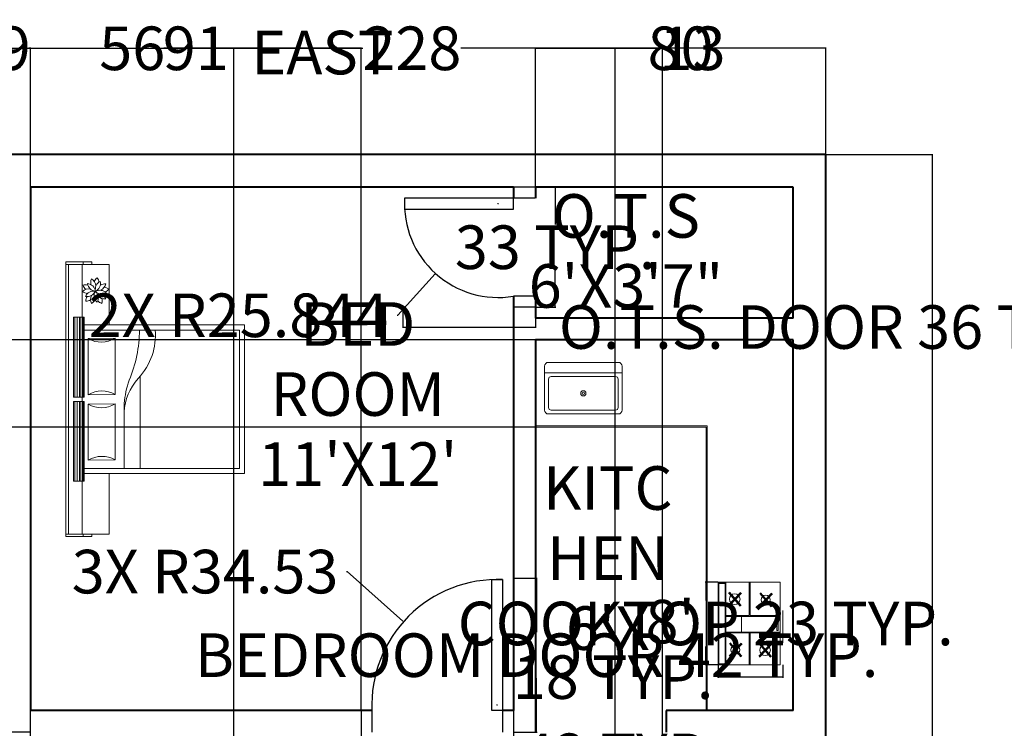
# Model space of a CAD drawing. Units: inches. Extents: x -124 to 612, y -69 to 524.
# Tile 6 of 9: x 16 to 287, y 329 to 524. Entities that reach past the tile are written whole.
import ezdxf
from ezdxf.enums import TextEntityAlignment as Align

# ---------------------------------------------------------------- set-up
doc = ezdxf.new("R2010")
doc.units = ezdxf.units.IN
doc.header["$MEASUREMENT"] = 0
for name, color, linetype, lineweight in [('A-ANNO-DIMS', 2, 'Continuous', 18), ('A-ANNO-TEXT', 1, 'Continuous', 18), ('A-AREA-IDEN', 1, 'Continuous', 18), ('A-DOOR', 4, 'Continuous', 25), ('A-EQPM', 9, 'Continuous', 18), ('A-FLOR-CASE', 8, 'Continuous', 18), ('A-FLOR-FIXT', 9, 'Continuous', 18), ('A-FURN', 8, 'Continuous', 18), ('A-WALL', 7, 'Continuous', 40)]:
    doc.layers.add(name, color=color, linetype=linetype, lineweight=lineweight)
doc.styles.add('ATTR', font='romans.shx', dxfattribs={"width": 0.8, "height": 1.075})
doc.styles.get("Standard").update_dxf_attribs({"font": 'arial.ttf'})
doc.dimstyles.get("Standard").update_dxf_attribs({"dimtxt": 12, "dimasz": 0.18, "dimexe": 0.18, "dimexo": 0.0625, "dimgap": 0.09, "dimtad": 0, "dimtih": 1, "dimtoh": 1, "dimdec": 0, "dimzin": 0, "dimdsep": 46, "dimlunit": 4, "dimtxsty": 'Standard', "dimcen": 0.09, "dimadec": 0, "dimazin": 0, "dimtfac": 1, "dimtdec": 0, "dimtofl": 0, "dimtmove": 0, "dimatfit": 3, "dimfxl": 1, "dimtolj": 1, "dimtzin": 0, "dimarcsym": 0})

# ---------------------------------------------------------------- blocks, each defined once
blk = doc.blocks.new('A$C7BDD1693')
for p, q in [((0, 2.068), (0, 1.768)), ((0, 2.068), (1.615, 2.068)), ((0.03, 1.768), (0.03, 2.068)), ((1.615, 2.068), (2.54, 2.068)), ((2.54, 2.068), (3.18, 2.068)), ((3.15, 1.768), (3.15, 2.068)), ((3.18, 2.068), (3.18, 1.768)), ((0.03, 2.038), (0.64, 2.038)), ((0.64, 2.038), (1.565, 2.038)), ((0.64, 1.978), (1.565, 1.978)), ((0.64, 1.978), (0.64, 1.858)), ((0.64, 1.963), (1.565, 1.963)), ((1.565, 2.038), (1.615, 2.038)), ((1.565, 1.978), (1.565, 1.858)), ((1.615, 2.038), (2.54, 2.038)), ((1.615, 1.978), (1.615, 1.858)), ((1.615, 1.978), (2.54, 1.978)), ((1.615, 1.963), (2.54, 1.963)), ((3.15, 2.038), (2.54, 2.038)), ((2.54, 1.978), (2.54, 1.858)), ((0.03, 1.868), (0, 1.868)), ((0.03, 1.88), (0.64, 1.88)), ((0.64, 1.937), (1.565, 1.937)), ((0.64, 1.912), (1.565, 1.912)), ((0.64, 1.893), (1.565, 1.893)), ((0.64, 1.877), (1.565, 1.877)), ((0.64, 1.866), (1.565, 1.866)), ((0.64, 1.858), (1.565, 1.858)), ((0.73, 1.568), (0.73, 1.858)), ((0.79, 1.858), (0.79, 0.06)), ((1.565, 1.88), (1.615, 1.88)), ((1.615, 1.937), (2.54, 1.937)), ((1.615, 1.912), (2.54, 1.912)), ((1.615, 1.893), (2.54, 1.893)), ((1.615, 1.877), (2.54, 1.877)), ((1.615, 1.866), (2.54, 1.866)), ((1.615, 1.858), (2.54, 1.858)), ((2.39, 1.858), (2.39, 0.06)), ((2.45, 1.568), (2.45, 1.858)), ((3.15, 1.88), (2.54, 1.88)), ((3.15, 1.868), (3.18, 1.868)), ((0, 1.768), (0.03, 1.768)), ((0.03, 1.768), (0.03, 1.568)), ((0.03, 1.768), (0.03, 1.568)), ((1.533, 1.81), (0.883, 1.81)), ((0.883, 1.81), (0.887, 1.498)), ((1.537, 1.498), (1.533, 1.81)), ((2.291, 1.81), (1.641, 1.81)), ((1.641, 1.81), (1.646, 1.498)), ((2.296, 1.498), (2.291, 1.81)), ((3.15, 1.568), (3.15, 1.768)), ((3.18, 1.768), (3.15, 1.768)), ((0.03, 1.568), (0.73, 1.568)), ((0.73, 1.568), (0.73, 0)), ((0.887, 1.498), (1.537, 1.498)), ((1.646, 1.498), (2.296, 1.498)), ((3.15, 1.568), (2.45, 1.568)), ((2.45, 1.568), (2.45, 0)), ((1.54, 1.392), (0.79, 1.392)), ((1.848, 1.209), (0.79, 1.209)), ((0.73, 0), (2.45, 0)), ((0.79, 0.06), (2.39, 0.06))]:
    blk.add_line(p, q)
for centre, radius, start, end in [((2.879, 1.849), 0.155, 184.2105, 205.3514), ((2.726, 1.74), 0.0968, 57.5086, 91.2476), ((2.884, 1.823), 0.106, 170.7761, 244.5159), ((2.743, 1.749), 0.098, 347.0447, 68.2473), ((2.938, 1.802), 0.125, 143.1301, 173.4932), ((2.751, 1.802), 0.115, 351.1324, 40.6013), ((2.967, 1.726), 0.155, 112.2105, 133.3514), ((2.817, 1.838), 0.0968, 345.5086, 19.2476), ((0.626, 1.65), 0.303, 329.8722, 31.8713), ((1.794, 1.658), 0.303, 149.8722, 211.8713), ((1.384, 1.65), 0.303, 329.8722, 31.8713), ((2.553, 1.658), 0.303, 149.8722, 211.8713), ((2.74, 1.667), 0.115, 63.1324, 112.6013), ((2.798, 1.845), 0.125, 215.1301, 245.4931), ((2.788, 1.643), 0.098, 59.0447, 140.2473), ((2.761, 1.8), 0.106, 242.7761, 316.5159), ((2.903, 1.653), 0.098, 131.0447, 212.2473), ((2.745, 1.676), 0.106, 314.7761, 28.5159), ((2.944, 1.713), 0.106, 98.7761, 172.5159), ((2.83, 1.825), 0.098, 275.0447, 356.2473), ((2.858, 1.622), 0.106, 26.7761, 100.5159), ((2.929, 1.765), 0.098, 203.0447, 284.2473), ((2.883, 1.833), 0.115, 279.1324, 328.6013), ((2.941, 1.655), 0.125, 71.1301, 101.4931), ((2.877, 1.605), 0.155, 40.2105, 61.3514), ((2.791, 1.624), 0.0968, 129.5086, 163.2476), ((2.735, 1.803), 0.155, 256.2105, 277.3514), ((2.865, 1.615), 0.115, 135.1324, 184.6013), ((2.713, 1.725), 0.125, 287.1301, 317.4932), ((2.921, 1.65), 0.0968, 201.5086, 235.2476), ((2.953, 1.718), 0.115, 207.1324, 256.6013), ((2.734, 1.652), 0.155, 328.2105, 349.3514), ((2.802, 1.607), 0.125, 359.1301, 29.4932), ((2.937, 1.782), 0.0968, 273.5086, 307.2476)]:
    blk.add_arc(centre, radius, start, end)
for centre, major_axis, ratio, start_param, end_param in [((1.413, 0.552), (0, -0.842), 0.84, 2.512571, 3.097265), ((1.474, 0.023), (0, -1.371), 0.84, 2.845884, 3.083884), ((2.394, 3.329), (0, -2.112), 0.84, -0.336035, -0.002349), ((2.261, 1.856), (0.259, -0.793), 0.868451, -0.988378, -0.183496)]:
    blk.add_ellipse(centre, major_axis=major_axis, ratio=ratio, start_param=start_param, end_param=end_param)
blk = doc.blocks.new('A$C0FBA78B1')
for p, q in [((749.7, 588.6), (0, 588.6)), ((0, 588.6), (0, 23.9)), ((0, 518.1), (0, 584.3)), ((0, 584.3), (744.6, 584.3)), ((7.1, 524.3), (7.1, 580.2)), ((7.1, 580.2), (737.6, 580.2)), ((737.6, 580.2), (737.6, 524.3)), ((744.6, 584.3), (744.6, 518.1)), ((749.7, 588.6), (749.7, 24)), ((744.6, 518.1), (0, 518.1)), ((737.6, 524.3), (7.1, 524.3)), ((70.4, 380.5), (191.9, 485.9)), ((189.2, 369.7), (72.8, 480.7)), ((74, 376.5), (195.5, 481.8)), ((192.9, 373.6), (76.6, 484.7)), ((77.5, 372.4), (199, 477.7)), ((196.6, 377.5), (80.3, 488.6)), ((288.9, 518.1), (288.9, 305)), ((295.8, 518.1), (295.8, 24)), ((438.8, 518.1), (438.8, 296.7)), ((446.5, 518.1), (446.5, 305.1)), ((531, 386.7), (652.5, 492.1)), ((649.8, 375.9), (533.4, 486.9)), ((534.6, 382.6), (656.1, 488)), ((653.5, 379.8), (537.1, 490.8)), ((538.1, 378.5), (659.6, 483.9)), ((657.2, 383.7), (540.9, 494.7)), ((295.8, 376.5), (438.1, 376.5)), ((0, 305), (288.9, 305)), ((0, 296.6), (288.9, 296.7)), ((288.9, 296.7), (288.9, 24)), ((438.8, 296.7), (438.8, 24)), ((446.5, 305.1), (749.7, 305.1)), ((446.5, 296.7), (446.5, 24)), ((446.5, 296.7), (749.7, 296.7)), ((67.4, 110.2), (188.9, 215.6)), ((186.2, 99.4), (69.8, 210.4)), ((71, 106.1), (192.5, 211.5)), ((189.9, 103.3), (73.5, 214.4)), ((74.5, 102.1), (196, 207.4)), ((193.6, 107.2), (77.3, 218.3)), ((525, 104.1), (646.5, 209.5)), ((643.7, 93.3), (527.3, 204.4)), ((528.5, 100.1), (650, 205.4)), ((647.4, 97.2), (531.1, 208.3)), ((532, 96), (653.5, 201.3)), ((651.2, 101.1), (534.8, 212.2)), ((0, 23.9), (749.7, 24)), ((494.5, 0), (198.4, 0)), ((311.1, 41.1), (311.1, 53.6)), ((311.1, 53.6), (424.4, 53.6)), ((424.4, 41.1), (311.1, 41.1)), ((424.4, 53.6), (424.4, 41.1))]:
    blk.add_line(p, q)
for centre, radius in [((135.8, 431.1), 41.2), ((596.4, 437.3), 48.4), ((132.8, 160.8), 48.4), ((590.3, 154.7), 41.2)]:
    blk.add_circle(centre, radius)
blk = doc.blocks.new("30'' Sink Single PV")
blk.add_line((-15, -3.999996), (15, -3.999996))
for points in [[(-13.5, 0), (13.5, 0)], [(-15, -18.499996), (-15, -1.5)], [(15, -1.5), (15, -18.499996)], [(-13.5, -17.499996), (-13.5, -6.499996)], [(-12.5, -5.499996), (12.5, -5.499996)], [(13.5, -6.499996), (13.5, -17.499996)], [(12.5, -18.499996), (-12.5, -18.499996)], [(13.5, -19.999996), (-13.5, -19.999996)]]:
    blk.add_lwpolyline(points)
for radius in [1, 0.5]:
    blk.add_circle((0, -11.999996), radius)
for centre, radius, start, end in [((-13.5, -1.5), 1.5, 90, 180), ((13.5, -1.5), 1.5, 0, 90), ((-12.5, -6.499996), 1, 90, 180), ((12.5, -6.499996), 1, 0, 90), ((-13.5, -18.499996), 1.5, 180, 270), ((-12.5, -17.499996), 1, 180, 270), ((12.5, -17.499996), 1, 270, 0), ((13.5, -18.499996), 1.5, 270, 0)]:
    blk.add_arc(centre, radius, start, end)
at = {"style": 'ATTR', "width": 0.8, "flags": 9}
blk.add_attdef('ESTCODE', (0, 0), '', height=0.006, dxfattribs=at)
blk = doc.blocks.new('DOOR-36IN-SINGLE')
for p, q in [((0, 6), (0, 0)), ((3, 6), (3, 0)), ((39, 6), (39, 0)), ((42, 6), (42, 0))]:
    blk.add_line(p, q)
blk.add_lwpolyline([(39, 6), (36, 6), (36, 42), (39, 42)], close=True)
blk.add_arc((37.5, 7.5), 34.53, 87.5104, 182.4896)
blk = doc.blocks.new('DOOR-30IN-OTS')
for p, q in [((36.04, 33), (30.04, 33)), ((36.04, 30), (30.04, 30)), ((36.04, 3), (30.04, 3)), ((36.04, 0), (30.04, 0))]:
    blk.add_line(p, q)
blk.add_lwpolyline([(30.04, 30), (0.04, 30), (0.04, 27), (30.04, 27)], close=True)
blk.add_arc((25.84, 28.5), 25.84, 176.6726, 279.353)
blk = doc.blocks.new('COUNTER-L-KITCHEN')
for p, q in [((47.3, 78.3), (0, 78.3)), ((47, 78), (0, 78)), ((47, 0), (47, 78)), ((47.3, 0), (47.3, 78.3))]:
    blk.add_line(p, q)
blk = doc.blocks.new('*D23')
at = {"layer": 'A-ANNO-DIMS', "color": 0, "lineweight": -2, "transparency": 16777216}
for p, q in [((152.41, 370.45), (158.89, 370.45)), ((158.71, 370.27), (158.71, 355.54)), ((158.71, 328.21), (158.71, 342.94)), ((152.41, 328.03), (158.89, 328.03))]:
    blk.add_line(p, q, dxfattribs=at)
at = {"layer": 'A-ANNO-DIMS', "color": 0, "transparency": 16777216}
for points in [[(158.68, 370.27), (158.74, 370.27), (158.71, 370.45)], [(158.68, 328.21), (158.74, 328.21), (158.71, 328.03)]]:
    blk.add_solid(points, dxfattribs=at)
at = {"layer": 'Defpoints', "color": 0, "transparency": 16777216}
for p in [(152.35, 370.45), (158.71, 370.45), (152.35, 328.03)]:
    blk.add_point(p, dxfattribs=at)
at = {"layer": 'A-ANNO-DIMS', "color": 0, "transparency": 16777216, "insert": (158.71, 349.24), "char_height": 12, "attachment_point": 5}
blk.add_mtext('\\A1;BEDROOM DOOR 42 TYP.', dxfattribs=at)
blk = doc.blocks.new('*D24')
at = {"layer": 'A-ANNO-DIMS', "color": 0, "lineweight": -2, "transparency": 16777216}
for p, q in [((110.35, 327.97), (110.35, 321.49)), ((152.35, 327.97), (152.35, 321.49)), ((110.53, 321.67), (152.17, 321.67)), ((152.35, 321.67), (152.53, 321.67))]:
    blk.add_line(p, q, dxfattribs=at)
at = {"layer": 'A-ANNO-DIMS', "color": 0, "transparency": 16777216}
for points in [[(110.53, 321.7), (110.53, 321.64), (110.35, 321.67)], [(152.17, 321.7), (152.17, 321.64), (152.35, 321.67)]]:
    blk.add_solid(points, dxfattribs=at)
at = {"layer": 'Defpoints', "color": 0, "transparency": 16777216}
for p in [(110.35, 328.03), (152.35, 328.03), (152.35, 321.67)]:
    blk.add_point(p, dxfattribs=at)
at = {"layer": 'A-ANNO-DIMS', "color": 0, "transparency": 16777216, "insert": (182.07, 321.67), "char_height": 12, "attachment_point": 5}
blk.add_mtext('\\A1;42 TYP.', dxfattribs=at)
blk = doc.blocks.new('*D31')
at = {"layer": 'A-ANNO-DIMS', "color": 0, "lineweight": -2, "transparency": 16777216}
for p, q in [((208.6, 369.3), (205.08, 369.3)), ((205.26, 369.12), (205.26, 364.26)), ((205.26, 346.8), (205.26, 351.66)), ((208.6, 346.62), (205.08, 346.62))]:
    blk.add_line(p, q, dxfattribs=at)
at = {"layer": 'A-ANNO-DIMS', "color": 0, "transparency": 16777216}
for points in [[(205.23, 369.12), (205.29, 369.12), (205.26, 369.3)], [(205.23, 346.8), (205.29, 346.8), (205.26, 346.62)]]:
    blk.add_solid(points, dxfattribs=at)
at = {"layer": 'Defpoints', "color": 0, "transparency": 16777216}
for p in [(205.26, 369.3), (208.66, 369.3), (208.66, 346.62)]:
    blk.add_point(p, dxfattribs=at)
at = {"layer": 'A-ANNO-DIMS', "color": 0, "transparency": 16777216, "insert": (205.26, 357.96), "char_height": 12, "attachment_point": 5}
blk.add_mtext('\\A1;COOKTOP 23 TYP.', dxfattribs=at)
blk = doc.blocks.new('*D32')
at = {"layer": 'A-ANNO-DIMS', "color": 0, "lineweight": -2, "transparency": 16777216}
for p, q in [((208.66, 346.55), (208.66, 343.03)), ((226.48, 346.55), (226.48, 343.03)), ((208.66, 343.21), (208.48, 343.21)), ((226.3, 343.21), (208.84, 343.21))]:
    blk.add_line(p, q, dxfattribs=at)
at = {"layer": 'A-ANNO-DIMS', "color": 0, "transparency": 16777216}
for points in [[(208.84, 343.24), (208.84, 343.18), (208.66, 343.21)], [(226.3, 343.24), (226.3, 343.18), (226.48, 343.21)]]:
    blk.add_solid(points, dxfattribs=at)
at = {"layer": 'Defpoints', "color": 0, "transparency": 16777216}
for p in [(208.66, 346.62), (226.48, 346.62), (208.66, 343.21)]:
    blk.add_point(p, dxfattribs=at)
at = {"layer": 'A-ANNO-DIMS', "color": 0, "transparency": 16777216, "insert": (179.75, 343.21), "char_height": 12, "attachment_point": 5}
blk.add_mtext('\\A1;18 TYP.', dxfattribs=at)
blk = doc.blocks.new('*D37')
at = {"layer": 'A-ANNO-DIMS', "color": 0, "lineweight": -2, "transparency": 16777216}
for p, q in [((121.9, 444.97), (121.9, 439.38)), ((158.35, 444.97), (158.35, 439.38)), ((122.08, 439.56), (158.17, 439.56)), ((158.35, 439.56), (158.53, 439.56))]:
    blk.add_line(p, q, dxfattribs=at)
at = {"layer": 'A-ANNO-DIMS', "color": 0, "transparency": 16777216}
for points in [[(122.08, 439.59), (122.08, 439.53), (121.9, 439.56)], [(158.17, 439.59), (158.17, 439.53), (158.35, 439.56)]]:
    blk.add_solid(points, dxfattribs=at)
at = {"layer": 'Defpoints', "color": 0, "transparency": 16777216}
for p in [(121.9, 445.03), (158.35, 445.03), (158.35, 439.56)]:
    blk.add_point(p, dxfattribs=at)
at = {"layer": 'A-ANNO-DIMS', "color": 0, "transparency": 16777216, "insert": (241.79, 439.56), "char_height": 12, "attachment_point": 5}
blk.add_mtext('\\A1;O.T.S. DOOR 36 TYP.', dxfattribs=at)
blk = doc.blocks.new('*D38')
at = {"layer": 'A-ANNO-DIMS', "color": 0, "lineweight": -2, "transparency": 16777216}
for p, q in [((158.41, 478.03), (164, 478.03)), ((163.82, 477.85), (163.82, 467.75)), ((163.82, 445.21), (163.82, 455.31)), ((158.41, 445.03), (164, 445.03))]:
    blk.add_line(p, q, dxfattribs=at)
at = {"layer": 'A-ANNO-DIMS', "color": 0, "transparency": 16777216}
for points in [[(163.79, 477.85), (163.85, 477.85), (163.82, 478.03)], [(163.79, 445.21), (163.85, 445.21), (163.82, 445.03)]]:
    blk.add_solid(points, dxfattribs=at)
at = {"layer": 'Defpoints', "color": 0, "transparency": 16777216}
for p in [(158.35, 478.03), (163.82, 478.03), (158.35, 445.03)]:
    blk.add_point(p, dxfattribs=at)
at = {"layer": 'A-ANNO-DIMS', "color": 0, "transparency": 16777216, "insert": (163.82, 461.53), "char_height": 12, "attachment_point": 5}
blk.add_mtext('\\A1;33 TYP.', dxfattribs=at)
blk = doc.blocks.new('*D47')
at = {"layer": 'A-ANNO-DIMS', "color": 0, "lineweight": -2, "transparency": 16777216}
for p, q in [((10.35, 487.09), (10.35, 516.46)), ((10.53, 516.28), (110.89, 516.28)), ((238.17, 516.28), (137.81, 516.28)), ((238.35, 487.09), (238.35, 516.46))]:
    blk.add_line(p, q, dxfattribs=at)
at = {"layer": 'A-ANNO-DIMS', "color": 0, "transparency": 16777216}
for points in [[(10.53, 516.31), (10.53, 516.25), (10.35, 516.28)], [(238.17, 516.31), (238.17, 516.25), (238.35, 516.28)]]:
    blk.add_solid(points, dxfattribs=at)
at = {"layer": 'Defpoints', "color": 0, "transparency": 16777216}
for p in [(238.35, 516.28), (10.35, 487.03), (238.35, 487.03)]:
    blk.add_point(p, dxfattribs=at)
at = {"layer": 'A-ANNO-DIMS', "color": 0, "transparency": 16777216, "insert": (124.35, 516.28), "char_height": 12, "attachment_point": 5}
blk.add_mtext('\\A1;228', dxfattribs=at)
blk = doc.blocks.new('*D48')
at = {"layer": 'A-ANNO-DIMS', "color": 0, "lineweight": -2, "transparency": 16777216}
for p, q in [((238.41, 487.03), (267.78, 487.03)), ((267.6, 486.85), (267.6, 253.25)), ((267.6, 7.21), (267.6, 240.81)), ((238.41, 7.03), (267.78, 7.03))]:
    blk.add_line(p, q, dxfattribs=at)
at = {"layer": 'A-ANNO-DIMS', "color": 0, "transparency": 16777216}
for points in [[(267.57, 486.85), (267.63, 486.85), (267.6, 487.03)], [(267.57, 7.21), (267.63, 7.21), (267.6, 7.03)]]:
    blk.add_solid(points, dxfattribs=at)
at = {"layer": 'Defpoints', "color": 0, "transparency": 16777216}
for p in [(238.35, 487.03), (267.6, 487.03), (238.35, 7.03)]:
    blk.add_point(p, dxfattribs=at)
at = {"layer": 'A-ANNO-DIMS', "color": 0, "transparency": 16777216, "insert": (267.6, 247.03), "char_height": 12, "attachment_point": 5}
blk.add_mtext('\\A1;480', dxfattribs=at)
blk = doc.blocks.new('*D51')
at = {"layer": 'A-ANNO-DIMS', "color": 0, "lineweight": -2, "transparency": 16777216}
for p, q in [((19.35, 196.09), (19.35, 516.46)), ((19.53, 516.28), (38.67, 516.28)), ((75.17, 516.28), (56.03, 516.28)), ((75.35, 196.09), (75.35, 516.46))]:
    blk.add_line(p, q, dxfattribs=at)
at = {"layer": 'A-ANNO-DIMS', "color": 0, "transparency": 16777216}
for points in [[(19.53, 516.31), (19.53, 516.25), (19.35, 516.28)], [(75.17, 516.31), (75.17, 516.25), (75.35, 516.28)]]:
    blk.add_solid(points, dxfattribs=at)
at = {"layer": 'Defpoints', "color": 0, "transparency": 16777216}
for p in [(75.35, 516.28), (19.35, 196.03), (75.35, 196.03)]:
    blk.add_point(p, dxfattribs=at)
at = {"layer": 'A-ANNO-DIMS', "color": 0, "transparency": 16777216, "insert": (47.35, 516.28), "char_height": 12, "attachment_point": 5}
blk.add_mtext('\\A1;56', dxfattribs=at)
blk = doc.blocks.new('*D53')
at = {"layer": 'A-ANNO-DIMS', "color": 0, "lineweight": -2, "transparency": 16777216}
for p, q in [((10.35, 487.09), (10.35, 516.46)), ((10.53, 516.28), (10.82, 516.28)), ((19.17, 516.28), (18.89, 516.28)), ((19.35, 478.09), (19.35, 516.46))]:
    blk.add_line(p, q, dxfattribs=at)
at = {"layer": 'A-ANNO-DIMS', "color": 0, "transparency": 16777216}
for points in [[(10.53, 516.31), (10.53, 516.25), (10.35, 516.28)], [(19.17, 516.31), (19.17, 516.25), (19.35, 516.28)]]:
    blk.add_solid(points, dxfattribs=at)
at = {"layer": 'Defpoints', "color": 0, "transparency": 16777216}
for p in [(10.35, 516.28), (10.35, 487.03), (19.35, 478.03)]:
    blk.add_point(p, dxfattribs=at)
at = {"layer": 'A-ANNO-DIMS', "color": 0, "transparency": 16777216, "insert": (14.85, 516.28), "char_height": 12, "attachment_point": 5}
blk.add_mtext('\\A1;9', dxfattribs=at)
blk = doc.blocks.new('*D57')
at = {"layer": 'A-ANNO-DIMS', "color": 0, "lineweight": -2, "transparency": 16777216}
for p, q in [((10.29, 487.03), (-19.08, 487.03)), ((-18.9, 486.85), (-18.9, 413.75)), ((-18.9, 328.21), (-18.9, 401.31)), ((19.29, 328.03), (-19.08, 328.03))]:
    blk.add_line(p, q, dxfattribs=at)
at = {"layer": 'A-ANNO-DIMS', "color": 0, "transparency": 16777216}
for points in [[(-18.93, 486.85), (-18.87, 486.85), (-18.9, 487.03)], [(-18.93, 328.21), (-18.87, 328.21), (-18.9, 328.03)]]:
    blk.add_solid(points, dxfattribs=at)
at = {"layer": 'Defpoints', "color": 0, "transparency": 16777216}
for p in [(-18.9, 487.03), (10.35, 487.03), (19.35, 328.03)]:
    blk.add_point(p, dxfattribs=at)
at = {"layer": 'A-ANNO-DIMS', "color": 0, "transparency": 16777216, "insert": (-18.9, 407.53), "char_height": 12, "attachment_point": 5}
blk.add_mtext('\\A1;159', dxfattribs=at)
blk = doc.blocks.new('*D65')
at = {"layer": 'A-ANNO-DIMS', "color": 0, "lineweight": -2, "transparency": 16777216}
for p, q in [((180.35, 112.09), (180.35, 516.46)), ((180.53, 516.28), (193.17, 516.28)), ((193.35, 112.09), (193.35, 516.46)), ((193.35, 516.28), (193.53, 516.28))]:
    blk.add_line(p, q, dxfattribs=at)
at = {"layer": 'A-ANNO-DIMS', "color": 0, "transparency": 16777216}
for points in [[(180.53, 516.31), (180.53, 516.25), (180.35, 516.28)], [(193.17, 516.31), (193.17, 516.25), (193.35, 516.28)]]:
    blk.add_solid(points, dxfattribs=at)
at = {"layer": 'Defpoints', "color": 0, "transparency": 16777216}
for p in [(193.35, 516.28), (180.35, 112.03), (193.35, 112.03)]:
    blk.add_point(p, dxfattribs=at)
at = {"layer": 'A-ANNO-DIMS', "color": 0, "transparency": 16777216, "insert": (201.65, 516.28), "char_height": 12, "attachment_point": 5}
blk.add_mtext('\\A1;13', dxfattribs=at)
blk = doc.blocks.new('*D67')
at = {"layer": 'A-ANNO-DIMS', "color": 0, "lineweight": -2, "transparency": 16777216}
for p, q in [((158.35, 478.09), (158.35, 516.46)), ((158.53, 516.28), (189.68, 516.28)), ((238.17, 516.28), (207.02, 516.28)), ((238.35, 487.09), (238.35, 516.46))]:
    blk.add_line(p, q, dxfattribs=at)
at = {"layer": 'A-ANNO-DIMS', "color": 0, "transparency": 16777216}
for points in [[(158.53, 516.31), (158.53, 516.25), (158.35, 516.28)], [(238.17, 516.31), (238.17, 516.25), (238.35, 516.28)]]:
    blk.add_solid(points, dxfattribs=at)
at = {"layer": 'Defpoints', "color": 0, "transparency": 16777216}
for p in [(238.35, 516.28), (238.35, 487.03), (158.35, 478.03)]:
    blk.add_point(p, dxfattribs=at)
at = {"layer": 'A-ANNO-DIMS', "color": 0, "transparency": 16777216, "insert": (198.35, 516.28), "char_height": 12, "attachment_point": 5}
blk.add_mtext('\\A1;80', dxfattribs=at)
blk = doc.blocks.new('*D70')
at = {"layer": 'A-ANNO-DIMS', "color": 0, "lineweight": -2, "transparency": 16777216}
for p, q in [((19.35, 334.09), (19.35, 516.46)), ((19.53, 516.28), (57.32, 516.28)), ((110.17, 516.28), (72.38, 516.28)), ((110.35, 334.09), (110.35, 516.46))]:
    blk.add_line(p, q, dxfattribs=at)
at = {"layer": 'A-ANNO-DIMS', "color": 0, "transparency": 16777216}
for points in [[(19.53, 516.31), (19.53, 516.25), (19.35, 516.28)], [(110.17, 516.31), (110.17, 516.25), (110.35, 516.28)]]:
    blk.add_solid(points, dxfattribs=at)
at = {"layer": 'Defpoints', "color": 0, "transparency": 16777216}
for p in [(110.35, 516.28), (19.35, 334.03), (110.35, 334.03)]:
    blk.add_point(p, dxfattribs=at)
at = {"layer": 'A-ANNO-DIMS', "color": 0, "transparency": 16777216, "insert": (64.85, 516.28), "char_height": 12, "attachment_point": 5}
blk.add_mtext('\\A1;91', dxfattribs=at)
blk = doc.blocks.new('*D71')
at = {"layer": 'A-ANNO-DIMS', "color": 0, "lineweight": -2, "transparency": 16777216}
for p, q in [((158.29, 436.03), (-19.08, 436.03)), ((-18.9, 435.85), (-18.9, 430.14)), ((-18.9, 412.21), (-18.9, 417.91)), ((158.29, 412.03), (-19.08, 412.03))]:
    blk.add_line(p, q, dxfattribs=at)
at = {"layer": 'A-ANNO-DIMS', "color": 0, "transparency": 16777216}
for points in [[(-18.93, 435.85), (-18.87, 435.85), (-18.9, 436.03)], [(-18.93, 412.21), (-18.87, 412.21), (-18.9, 412.03)]]:
    blk.add_solid(points, dxfattribs=at)
at = {"layer": 'Defpoints', "color": 0, "transparency": 16777216}
for p in [(-18.9, 436.03), (158.35, 436.03), (158.35, 412.03)]:
    blk.add_point(p, dxfattribs=at)
at = {"layer": 'A-ANNO-DIMS', "color": 0, "transparency": 16777216, "insert": (-18.9, 424.03), "char_height": 12, "attachment_point": 5}
blk.add_mtext('\\A1;24', dxfattribs=at)
blk = doc.blocks.new('*D73')
at = {"layer": 'A-ANNO-DIMS', "color": 0, "lineweight": -2, "transparency": 16777216}
for p, q in [((106.38, 372.24), (106.56, 372.24)), ((106.56, 372.24), (121.91, 358.59)), ((147.76, 335.53), (147.94, 335.53)), ((147.85, 335.44), (147.85, 335.62))]:
    blk.add_line(p, q, dxfattribs=at)
at = {"layer": 'A-ANNO-DIMS', "color": 0, "transparency": 16777216}
blk.add_solid([(121.93, 358.62), (121.89, 358.57), (122.04, 358.47)], dxfattribs=at)
at = {"layer": 'Defpoints', "color": 0, "transparency": 16777216}
for p in [(122.04, 358.47), (147.85, 335.53)]:
    blk.add_point(p, dxfattribs=at)
at = {"layer": 'A-ANNO-DIMS', "color": 0, "transparency": 16777216, "insert": (67.41, 372.24), "char_height": 12, "attachment_point": 5}
blk.add_mtext('\\A1;3X R34.53', dxfattribs=at)
blk = doc.blocks.new('*D74')
at = {"layer": 'A-ANNO-DIMS', "color": 0, "lineweight": -2, "transparency": 16777216}
for p, q in [((148.06, 473.53), (148.24, 473.53)), ((148.15, 473.44), (148.15, 473.62)), ((120.49, 442.79), (130.74, 454.19)), ((120.31, 442.79), (120.49, 442.79))]:
    blk.add_line(p, q, dxfattribs=at)
at = {"layer": 'A-ANNO-DIMS', "color": 0, "transparency": 16777216}
blk.add_solid([(130.72, 454.21), (130.76, 454.17), (130.86, 454.32)], dxfattribs=at)
at = {"layer": 'Defpoints', "color": 0, "transparency": 16777216}
for p in [(148.15, 473.53), (130.86, 454.32)]:
    blk.add_point(p, dxfattribs=at)
at = {"layer": 'A-ANNO-DIMS', "color": 0, "transparency": 16777216, "insert": (76.6, 442.79), "char_height": 12, "attachment_point": 5}
blk.add_mtext('\\A1;2X R25.844', dxfattribs=at)

msp = doc.modelspace()

# ---------------------------------------------------------------- linework, layer by layer
at = {"layer": 'A-WALL'}
for p, q in [((19.3513, 478.0291), (19.3513, 334.0291)), ((152.3513, 478.0291), (19.3513, 478.0291)), ((152.3513, 478.0291), (152.3513, 475.0291)), ((229.3513, 478.0291), (158.3513, 478.0291)), ((158.3513, 478.0291), (158.3513, 475.0291)), ((229.3513, 442.0291), (229.3513, 478.0291)), ((152.3513, 448.0291), (152.3513, 334.0291)), ((158.3513, 448.0291), (158.3513, 442.0291)), ((229.3513, 442.0291), (158.3513, 442.0291)), ((229.3513, 436.0291), (158.3513, 436.0291)), ((158.3513, 436.0291), (158.3513, 334.0291)), ((229.3513, 334.0291), (229.3513, 436.0291)), ((113.3513, 334.0291), (19.3513, 334.0291)), ((152.3513, 334.0291), (149.3513, 334.0291)), ((158.3513, 334.0291), (158.3513, 328.0291)), ((229.3513, 334.0291), (194.3513, 334.0291)), ((194.3513, 334.0291), (194.3513, 328.0291))]:
    msp.add_line(p, q, dxfattribs=at)
msp.add_lwpolyline([(10.3513, 7.0291), (238.3513, 7.0291), (238.3513, 487.0291), (10.3513, 487.0291)], close=True, dxfattribs=at)

# ---------------------------------------------------------------- block references
at = {"layer": 'A-DOOR'}
for name, p in [('DOOR-30IN-OTS', (122.308, 445.029)), ('DOOR-36IN-SINGLE', (110.351, 328.029))]:
    msp.add_blockref(name, p, dxfattribs=at)
at = {"layer": 'A-EQPM', "xscale": 0.030262411053157, "yscale": 0.030262411053157, "zscale": 0.030262411053157, "rotation": 90}
msp.add_blockref('A$C0FBA78B1', (226.4757, 346.6153), dxfattribs=at)
at = {"layer": 'A-FLOR-CASE'}
msp.add_blockref('COUNTER-L-KITCHEN', (158.351, 334.029), dxfattribs=at)
at = {"layer": 'A-FLOR-FIXT', "xscale": 0.710634528886296, "yscale": 0.710634528886296, "zscale": 0.710634528886296}
msp.add_blockref("30'' Sink Single PV", (171.5674, 429.8394, 10.4529), dxfattribs=at)
at = {"layer": 'A-FURN', "xscale": 23.78825355168716, "yscale": 23.78825355168716, "zscale": 23.78825355168716, "rotation": 90}
msp.add_blockref('A$C7BDD1693', (78.2769, 381.8673), dxfattribs=at)

# ---------------------------------------------------------------- texts
at = {"layer": 'A-ANNO-TEXT'}
msp.add_text('EAST', height=12, dxfattribs=at).set_placement((99.7039, 509.1109), align=Align.CENTER)
at = {"layer": 'A-AREA-IDEN'}
for s, p in [('O.T.S', (183.2809, 464.1392)), ('6\'X3\'7"', (183.2809, 444.8623)), ('BED', (109.4573, 434.3882)), ('ROOM', (109.4573, 415.1112)), ("11'X12'", (109.4573, 395.8343)), ('KITC', (178.2932, 389.2456)), ('HEN', (178.2932, 369.9686)), ("6'X", (178.2932, 350.6917)), ("8'", (195.5029, 352.4689))]:
    msp.add_text(s, height=12, dxfattribs=at).set_placement(p, align=Align.CENTER)

# ---------------------------------------------------------------- dimensions: what is measured, and where the dimension line sits
at = {"layer": 'A-ANNO-DIMS'}
for base, p1, p2, picture, middle in [((10.3513, 516.2791), (19.3513, 478.0291), (10.3513, 487.0291), '*D53', (14.8513, 516.2791)), ((238.3513, 516.2791), (10.3513, 487.0291), (238.3513, 487.0291), '*D47', (124.3513, 516.2791)), ((75.3513, 516.2791), (19.3513, 196.0291), (75.3513, 196.0291), '*D51', (47.3513, 516.2791)), ((110.3513, 516.2791), (19.3513, 334.0291), (110.3513, 334.0291), '*D70', (64.8513, 516.2791)), ((238.3513, 516.2791), (158.3513, 478.0291), (238.3513, 487.0291), '*D67', (198.3513, 516.2791)), ((193.3513, 516.2791), (180.3513, 112.0291), (193.3513, 112.0291), '*D65', (201.6513, 516.2791))]:
    dim = msp.add_linear_dim(base=base, p1=p1, p2=p2, dimstyle='Standard', override={"dimdec": 0, "dimlfac": 1, "dimrnd": 0, "dimzin": 0, "dimdsep": 46, "dimlunit": 2}, dxfattribs=at)
    dim.commit()
    dim.dimension.update_dxf_attribs({"geometry": picture, "text_midpoint": middle})
for base, p1, p2, picture, middle in [((-18.8987, 487.0291), (19.3513, 328.0291), (10.3513, 487.0291), '*D57', (-18.8987, 407.5291)), ((267.6013, 487.0291), (238.3513, 7.0291), (238.3513, 487.0291), '*D48', (267.6013, 247.0291)), ((-18.8987, 436.0291), (158.3513, 412.0291), (158.3513, 436.0291), '*D71', (-18.8987, 424.0291))]:
    dim = msp.add_linear_dim(base=base, p1=p1, p2=p2, angle=90, dimstyle='Standard', override={"dimdec": 0, "dimlfac": 1, "dimrnd": 0, "dimzin": 0, "dimdsep": 46, "dimlunit": 2}, dxfattribs=at)
    dim.commit()
    dim.dimension.update_dxf_attribs({"geometry": picture, "text_midpoint": middle})
for base, p1, p2, text, picture, middle in [((158.3513, 439.5607), (121.8956, 445.0291), (158.3513, 445.0291), 'O.T.S. DOOR <> TYP.', '*D37', (241.7905, 439.5607)), ((152.3513, 321.666), (110.3513, 328.0291), (152.3513, 328.0291), '<> TYP.', '*D24', (182.0688, 321.666))]:
    dim = msp.add_linear_dim(base=base, p1=p1, p2=p2, text=text, dimstyle='Standard', override={"dimdec": 0, "dimlfac": 1, "dimrnd": 0, "dimzin": 0, "dimdsep": 46, "dimlunit": 2}, dxfattribs=at)
    dim.commit()
    dim.dimension.update_dxf_attribs({"geometry": picture, "text_midpoint": middle})
for base, p1, p2, angle, text, picture, middle in [((163.8196, 478.0291), (158.3513, 445.0291), (158.3513, 478.0291), 90, '<> TYP.', '*D38', (163.8196, 461.5291)), ((158.7144, 370.4495), (152.3513, 328.0291), (152.3513, 370.4495), 90, 'BEDROOM DOOR <> TYP.', '*D23', (158.7144, 349.2393)), ((205.2604, 369.304), (208.6637, 346.6153), (208.6637, 369.304), 90, 'COOKTOP <> TYP.', '*D31', (205.2604, 357.9597)), ((208.6637, 343.2121), (226.4757, 346.6153), (208.6637, 346.6153), 180, '<> TYP.', '*D32', (179.7525, 343.2121))]:
    dim = msp.add_linear_dim(base=base, p1=p1, p2=p2, angle=angle, text=text, dimstyle='Standard', override={"dimdec": 0, "dimlfac": 1, "dimrnd": 0, "dimzin": 0, "dimdsep": 46, "dimlunit": 2}, dxfattribs=at)
    dim.commit()
    dim.dimension.update_dxf_attribs({"geometry": picture, "text_midpoint": middle})
for center, mpoint, text, override, picture, middle in [((148.1513, 473.5291), (130.8628, 454.3198), '2X <>', {"dimdec": 3, "dimlfac": 1, "dimrnd": 0, "dimzin": 0, "dimdsep": 46, "dimlunit": 2}, '*D74', (76.5989, 442.7942)), ((147.8513, 335.5291), (122.0433, 358.4735), '3X <>', {"dimdec": 2, "dimlfac": 1, "dimrnd": 0, "dimzin": 0, "dimdsep": 46, "dimlunit": 2}, '*D73', (67.4113, 372.2402))]:
    dim = msp.add_radius_dim(center=center, mpoint=mpoint, text=text, dimstyle='Standard', override=override, dxfattribs=at)
    dim.commit()
    dim.dimension.update_dxf_attribs({"geometry": picture, "text_midpoint": middle, "dimtype": 164})

doc.saveas('drawing.dxf')
